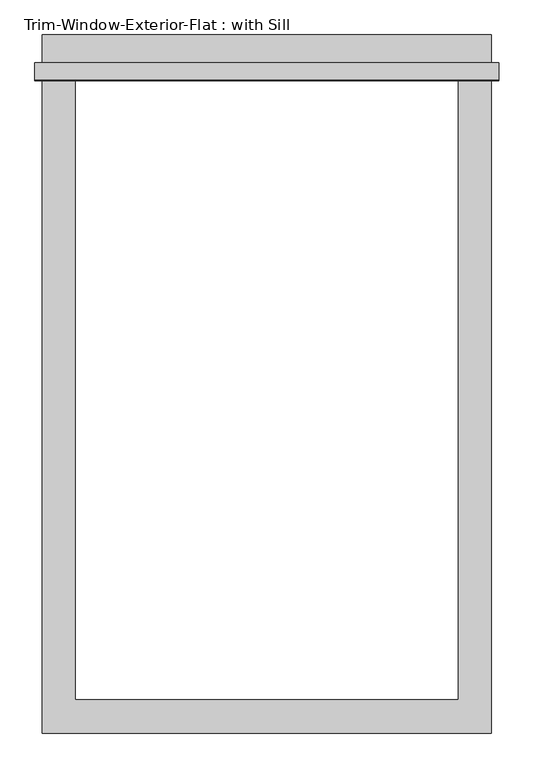
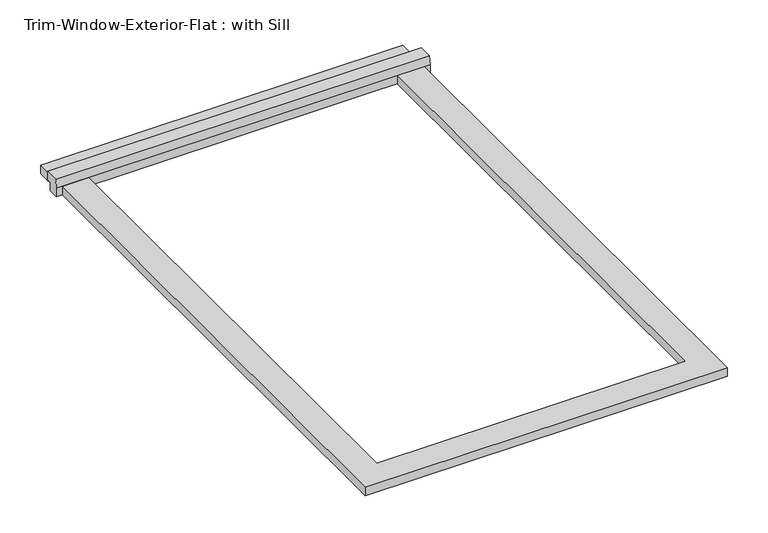
"""IFC4 building model written with IfcOpenShell, lengths in millimetres: proxy geometry, Trim-Window-Exterior-Flat : with Sill."""

from ifc_helpers import new_model, si_unit, frame, origin, origin_with_axes, place, context, project, spatial, polyline, outline, extrude, source, transform, mapped, element, save


def trim_window_exterior_flat_with_sill_5e960bf5(model_context):
    return source(origin(), model_context, "Body", "SweptSolid", [
        extrude(outline(polyline([(387.35, 1088.9823709), (-387.35, 1088.9823709), (-387.35, 1146.1323709), (387.35, 1146.1323709), (387.35, 1088.9823709)])), origin_with_axes(), (0.0, 0.0, 1.0), 19.05),
        extrude(outline(polyline([(1098.55, 38.1), (1098.55, 19.05), (1088.9823709, 19.05), (1088.9823709, 0.0), (1066.8, 0.0), (1066.8, 19.05), (1069.2580645, 38.1), (1098.55, 38.1)])), frame((-400.05, 0.0, 0.0), z_axis=(1.0, 0.0, 0.0), x_axis=(0.0, 1.0, 0.0)), (0.0, 0.0, 1.0), 800.1),
        extrude(outline(polyline([(-387.35, -57.15), (-387.35, 1066.8), (-330.2, 1066.8), (-330.2, 0.0), (330.2, 0.0), (330.2, 1066.8), (387.35, 1066.8), (387.35, -57.15), (-387.35, -57.15)])), origin_with_axes(), (0.0, 0.0, 1.0), 19.05),
    ])


if __name__ == "__main__":
    model = new_model("IFC4")
    model_context = context("Model", 3, world=origin())
    ifc_project = project(units=[si_unit("LENGTHUNIT", "METRE", prefix="MILLI")], contexts=[model_context])
    site = spatial("IfcSite", under=ifc_project)
    building = spatial("IfcBuilding", under=site)
    placement = place(None, origin())
    trim_window_exterior_flat_with_sill_shape = trim_window_exterior_flat_with_sill_5e960bf5(model_context)
    element("IfcBuildingElementProxy", 1, Name="Trim-Window-Exterior-Flat : with Sill", ObjectType="Trim-Window-Exterior-Flat : with Sill", at=placement, inside=building, context=model_context, shape_type="MappedRepresentation", body=[
        mapped(trim_window_exterior_flat_with_sill_shape, transform((0.0, 0.0, 0.0), x_axis=(1.0, 0.0, 0.0), y_axis=(0.0, 1.0, 0.0), z_axis=(0.0, 0.0, 1.0))),
    ])
    save(model, "model.ifc")

# Revit data of these elements
# Type "Trim-Window-Exterior-Flat : with Sill"
#   Trim Width = 0' - 2 1/4"
#   Trim Thickness_Picture Frame = 0' - 1 1/4"
#   Trim Thickness_with Sill = 0' - 0 3/4"
#   Sill Thickness = 0' - 1 1/4"
#   Opening Width [instance default] = 2' - 0"
#   Opening Height [instance default] = 3' - 0"
#   Default Elevation = 4' - 0"
#   Sill = yes
#   Picture Frame = no
#   Trim Material [instance default] = none
# Element 1 (IfcBuildingElementProxy, "Trim-Window-Exterior-Flat : with Sill")
#   Opening Width = 2' - 2"
#   Opening Height = 3' - 6"
#   Trim Material = Clad - White
#   Materials on its faces: "Clad - White"
# Materials
#   "Clad - White": class "Wood", colour RGB 242 242 238, transparency 0, Cost = 0
